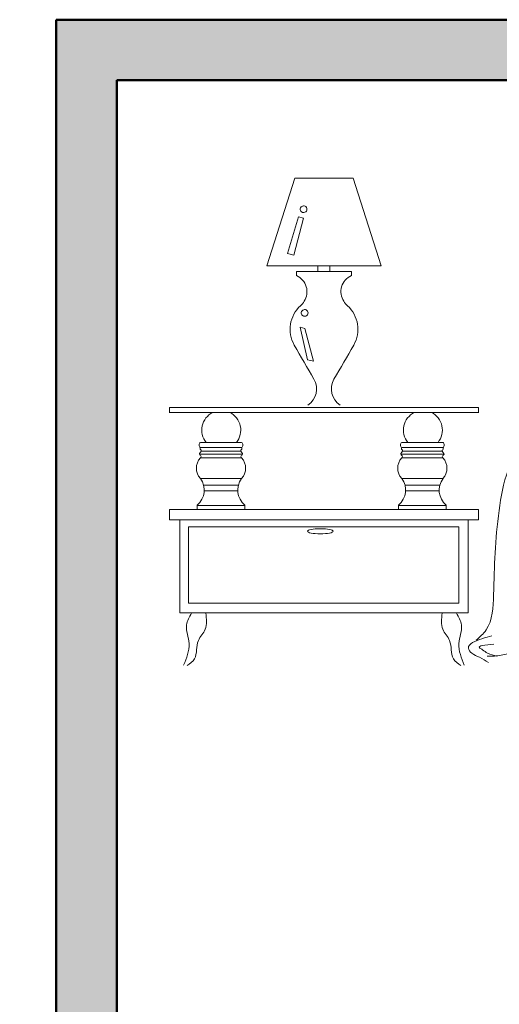
# Model space of a CAD drawing. Units: inches. Extents: x 1771 to 3025, y 319 to 889.
# Tile 9 of 35: x 1939 to 1978, y 713 to 795. Entities that reach past the tile are written whole.
import ezdxf

# ---------------------------------------------------------------- set-up
doc = ezdxf.new("R2010")
doc.units = ezdxf.units.IN
doc.header["$MEASUREMENT"] = 0
for name, color, linetype, lineweight in [('A-FURN', 8, 'Continuous', 18), ('A-WALL', 7, 'Continuous', 50), ('A-WALL-PATT', 254, 'Continuous', 13)]:
    doc.layers.add(name, color=color, linetype=linetype, lineweight=lineweight)

# ---------------------------------------------------------------- blocks, each defined once
blk = doc.blocks.new('A$C3F6F0378')
for p, q in [((188.6, 774.2), (242.7, 943.6)), ((356.2, 943.6), (242.7, 943.6)), ((410.4, 774.2), (356.2, 943.6)), ((229, 797.8), (250.3, 869.3)), ((259.4, 866.2), (241.2, 794.8)), ((250.3, 869.3), (259.4, 866.2)), ((241.2, 794.8), (229, 797.8)), ((410.4, 774.2), (188.6, 774.2)), ((246.2, 763), (246.2, 755.2)), ((246.2, 763), (246.2, 755.2)), ((352.5, 763), (246.2, 763)), ((287.7, 774.2), (287.7, 763)), ((311, 763), (287.7, 763)), ((311, 774.2), (311, 763)), ((352.5, 763), (352.5, 755.2)), ((352.5, 763), (352.5, 755.2)), ((253.5, 655.6), (262.6, 652.5)), ((267.2, 592.3), (253.5, 655.6)), ((262.6, 652.5), (279.4, 589.2)), ((279.4, 589.2), (267.2, 592.3)), ((598.4, 500), (0, 500)), ((0, 499.7), (0, 489.7)), ((598.4, 499.7), (598.4, 489.7)), ((598.4, 490), (0, 490)), ((140, 432.2), (60, 432.2)), ((140, 432.2), (60, 432.2)), ((140, 422.2), (60, 422.2)), ((529.9, 432.2), (449.9, 432.2)), ((529.9, 432.2), (449.9, 432.2)), ((529.9, 422.2), (449.9, 422.2)), ((141.9, 409.3), (58.1, 409.3)), ((140, 402.2), (60, 402.2)), ((138.2, 415.4), (61.8, 415.4)), ((531.8, 409.3), (447.9, 409.3)), ((529.9, 402.2), (449.9, 402.2)), ((528.1, 415.4), (451.7, 415.4)), ((140, 362.2), (60, 362.2)), ((133.7, 349.2), (66.3, 349.2)), ((529.9, 362.2), (449.9, 362.2)), ((523.5, 349.2), (456.2, 349.2)), ((132.4, 338.7), (67.5, 338.7)), ((522.3, 338.7), (457.4, 338.7)), ((53.7, 311), (53.7, 302.2)), ((146.3, 310.3), (53.7, 310.3)), ((146.3, 311), (146.3, 302.2)), ((443.6, 311), (443.6, 302.2)), ((536.1, 310.3), (443.6, 310.3)), ((536.1, 311), (536.1, 302.2)), ((0, 302.2), (0, 282.2)), ((598.4, 302.2), (0, 302.2)), ((80, 302.2), (120, 302.2)), ((80, 302.2), (130, 302.2)), ((469.9, 302.2), (509.9, 302.2)), ((469.9, 302.2), (519.9, 302.2)), ((598.4, 282.2), (598.4, 302.2)), ((598.4, 282.2), (0, 282.2)), ((20, 282.2), (20, 102.2)), ((37.2, 268.9), (560.2, 268.9)), ((37.2, 120.8), (37.2, 268.9)), ((560.2, 268.9), (560.2, 120.8)), ((578.4, 102.2), (578.4, 282.2)), ((560.2, 120.8), (37.2, 120.8)), ((20, 102.2), (578.4, 102.2))]:
    blk.add_line(p, q)
for centre, radius, start, end in [((259.7, 883.6), 6.48, 168.6084, 233.2112), ((259.7, 883.6), 6.49, 104.0344, 168.6084), ((259.6, 883.5), 6.42, 233.2112, 255.9722), ((260, 883.6), 6.51, 78.6968, 107.1924), ((259.7, 883.8), 6.69, 255.9722, 278.2688), ((259.7, 883.9), 6.81, 278.2688, 342.9026), ((260, 883.7), 6.5, 50.1648, 78.6968), ((260.1, 883.8), 6.35, 342.9026, 50.1648), ((232.6, 724.1), 33.9, 326.6744, 66.3416), ((366.1, 724.1), 33.9, 113.6584, 213.3256), ((231, 722.3), 34.4, 312.0366, 330.6067), ((367.7, 722.3), 34.4, 209.3933, 227.9634), ((295.2, 651.2), 61.5, 132.0366, 209.8723), ((261.7, 682.8), 6.49, 104.0344, 168.6084), ((262, 682.9), 6.51, 78.6968, 107.1924), ((262, 682.9), 6.5, 50.1648, 78.6968), ((262.1, 683), 6.35, 342.9026, 50.1648), ((303.6, 651.2), 61.5, 330.1277, 47.9634), ((261.7, 682.8), 6.48, 168.6084, 233.2112), ((261.6, 682.8), 6.42, 233.2112, 255.9722), ((261.7, 683), 6.69, 255.9722, 278.2688), ((261.7, 683.1), 6.81, 278.2688, 342.9026), ((9112.8, 5715.8), 10230.1, 209.87228, 210.29853), ((-8514, 5715.8), 10230.1, 329.70147, 330.12772), ((247.8, 535.9), 37.3, 302.5427, 30.2985), ((350.9, 535.9), 37.3, 149.7015, 237.4573), ((100.5, 456.1), 37.8, 115.9414, 219.2084), ((100.5, 456.1), 37.8, 320.7916, 64.0586), ((490.9, 456.1), 37.8, 115.9414, 219.2084), ((490.9, 456.1), 37.8, 320.7916, 64.0586), ((63.7, 427.2), 6.24, 126.78, 233.22), ((136.2, 427.2), 6.24, 306.78, 53.22), ((453.6, 427.2), 6.24, 126.78, 233.22), ((526.1, 427.2), 6.24, 306.78, 53.22), ((82, 382.2), 29.7, 137.7452, 222.2548), ((118, 382.2), 29.7, 317.7452, 42.2548), ((471.9, 382.2), 29.7, 137.7452, 222.2548), ((507.8, 382.2), 29.7, 317.7452, 42.2548), ((30.6, 339.8), 37, 308.7547, 37.2668), ((169.4, 339.8), 37, 142.7332, 231.2453), ((420.5, 339.8), 37, 308.7547, 37.2668), ((559.3, 339.8), 37, 142.7332, 231.2453)]:
    blk.add_arc(centre, radius, start, end)
blk.add_ellipse((292.3, 260.1), major_axis=(25, 0), ratio=0.2)
at = {"ltscale": 5}
for points, knots in [([(594.1, 49), (601.1, 55.3), (626, 78.1), (628.7, 172), (631.8, 287.1), (663.1, 436.6), (808.3, 475), (1037.5, 455.3), (1227.9, 458.5), (1322.1, 461.7)], [0, 0, 0, 0, 28.320233, 100.953775, 269.820348, 420.691469, 489.161544, 656.134073, 940.569207, 940.569207, 940.569207, 940.569207]), ([(624.2, 57.4), (618.3, 55.8), (603.1, 51.8), (572.2, 40.6), (586.5, 21.1), (602, 16.6), (612.3, 9.7), (617.8, 5.9)], [0, 0, 0, 0, 19.937155, 51.57724, 63.193909, 80.21631, 100.09061, 100.09061, 100.09061, 100.09061]), ([(628, 41.8), (612, 40.1), (592.4, 38.1), (608.5, 29.7), (617.4, 21.9), (627.8, 19.8), (634.3, 18.4)], [0, 0, 0, 0, 28.05485, 34.289435, 45.980108, 65.027556, 65.027556, 65.027556, 65.027556]), ([(615.5, 18.4), (620.3, 18.3), (633.7, 17.9), (664.9, 24.9), (717, 41.9), (776.4, 46.5), (816.6, 50.9), (832.8, 53.1), (835.5, 51), (835.9, 50.7)], [0, 0, 0, 0, 14.447875, 40.468341, 96.220884, 181.018327, 216.046098, 224.609189, 226.185962, 226.185962, 226.185962, 226.185962])]:
    blk.add_open_spline(points, degree=3, knots=knots, dxfattribs=at)
for points, knots in [([(60, 422.2), (59.5, 421), (58.6, 418.8), (63.4, 417.1), (60.1, 412.9), (56.2, 408.7), (63.1, 405.7), (60.8, 403.1), (60, 402.2)], [0, 0, 0, 0, 3.125, 6.207289, 10.622222, 14.901958, 20.470919, 23.596268, 23.596268, 23.596268, 23.596268]), ([(140, 422.2), (140.5, 421), (141.4, 418.8), (136.6, 417.1), (139.8, 412.9), (143.7, 408.7), (136.9, 405.7), (139.2, 403.1), (140, 402.2)], [0, 0, 0, 0, 3.125, 6.207289, 10.622222, 14.901958, 20.470919, 23.596268, 23.596268, 23.596268, 23.596268]), ([(449.9, 422.2), (449.4, 421), (448.5, 418.8), (453.2, 417.1), (450, 412.9), (446.1, 408.7), (453, 405.7), (450.7, 403.1), (449.9, 402.2)], [0, 0, 0, 0, 3.125, 6.207289, 10.622222, 14.901958, 20.470919, 23.596268, 23.596268, 23.596268, 23.596268]), ([(529.8, 422.2), (530.3, 421), (531.3, 418.8), (526.5, 417.1), (529.7, 412.9), (533.6, 408.7), (526.8, 405.7), (529, 403.1), (529.8, 402.2)], [0, 0, 0, 0, 3.125, 6.207289, 10.622222, 14.901958, 20.470919, 23.596268, 23.596268, 23.596268, 23.596268]), ([(42.9, 101.6), (38.6, 94.2), (28.1, 75.7), (43.8, 40.1), (33.3, 14.7), (27.7, 0.9)], [0, 0, 0, 0, 24.696996, 61.099524, 104.177437, 104.177437, 104.177437, 104.177437]), ([(70.4, 101.6), (71.9, 90.6), (74.7, 70.5), (49.8, 47.4), (55.7, 15.4), (39.9, 4), (34.3, 0)], [0, 0, 0, 0, 31.35672, 56.935761, 92.890491, 112.386558, 112.386558, 112.386558, 112.386558]), ([(528.3, 101.6), (526.8, 90.6), (524.1, 70.5), (549, 47.4), (543, 15.4), (558.9, 4), (564.5, 0)], [0, 0, 0, 0, 31.35672, 56.935761, 92.890491, 112.386558, 112.386558, 112.386558, 112.386558]), ([(555.9, 101.6), (560.2, 94.2), (570.6, 75.7), (554.9, 40.1), (565.4, 14.7), (571.1, 0.9)], [0, 0, 0, 0, 24.696996, 61.099524, 104.177437, 104.177437, 104.177437, 104.177437])]:
    blk.add_open_spline(points, degree=3, knots=knots)

msp = doc.modelspace()

# ---------------------------------------------------------------- hatches: boundary and pattern name
at = {"layer": 'A-WALL-PATT'}
h = msp.add_hatch(color=256, dxfattribs=at)
h.dxf.hatch_style = 1
h.paths.add_polyline_path([(1870.724, 888.634), (1799.724, 888.634), (1799.724, 878.634), (1870.724, 878.634)])
h.paths.add_polyline_path([(1968.767, 888.634), (1918.724, 888.634), (1918.724, 878.634), (1941.724, 878.634), (1941.724, 830.634), (1946.724, 830.634), (1946.724, 878.634), (1968.767, 878.634)])
h.paths.add_polyline_path([(2059.676, 888.634), (2016.767, 888.634), (2016.767, 878.634), (2037.724, 878.634), (2037.724, 794.634), (1941.724, 794.634), (1941.724, 758.634), (1941.724, 664.634), (1946.724, 664.634), (1946.724, 712), (1946.724, 789.634), (2054.724, 789.634), (2054.724, 794.634), (2042.325, 794.634), (2042.325, 798.62), (2042.325, 835.497), (2042.724, 878.634), (2059.676, 878.634)])
h.paths.add_polyline_path([(2100.724, 888.634), (2077.676, 888.634), (2077.676, 878.634), (2090.724, 878.634), (2090.724, 789.634), (2090.724, 768.608), (2100.724, 768.608)])
h.paths.add_polyline_path([(2100.724, 720.608), (2090.724, 720.608), (2090.724, 669.634), (1982.724, 669.634), (1982.724, 664.634), (2001.724, 664.634), (2001.724, 652.634), (2006.724, 652.634), (2006.724, 664.634), (2049.518, 664.634, -0.385549), (2050.522, 664.634), (2090.724, 664.634), (2090.724, 649.173), (2100.724, 649.173)])
edge = h.paths.add_edge_path()
edge.add_line((2100.724, 631.173), (2090.724, 631.173))
edge.add_line((2090.724, 631.173), (2090.724, 616.634))
edge.add_line((2090.724, 616.634), (2001.724, 616.634))
edge.add_line((2001.724, 616.634), (1982.724, 616.634))
edge.add_line((1982.724, 616.634), (1982.724, 611.634))
edge.add_line((1982.724, 611.634), (2024.672, 611.634))
edge.add_spline(control_points=[(2024.672, 611.634), (2027.581, 612.871), (2030.014, 613.313), (2032.469, 613.716)], knot_values=[484.321569, 484.321569, 484.321569, 484.321569, 625.498764, 625.498764, 625.498764, 625.498764], degree=3, periodic=0)
edge.add_line((2032.469, 613.716), (2033.205, 613.716))
edge.add_spline(control_points=[(2033.205, 613.716), (2035.66, 613.313), (2039.461, 612.871), (2042.204, 611.634)], knot_values=[484.321569, 484.321569, 484.321569, 484.321569, 625.498764, 625.498764, 625.498764, 625.498764], degree=3, periodic=0)
edge.add_line((2042.204, 611.634), (2090.724, 611.634))
edge.add_line((2090.724, 611.634), (2090.724, 581.106))
edge.add_line((2090.724, 581.106), (2100.724, 581.106))
edge.add_line((2100.724, 581.106), (2100.724, 631.173))
h.paths.add_polyline_path([(2100.724, 533.106), (2090.724, 533.106), (2090.724, 479.634), (1946.724, 479.634), (1946.724, 616.634), (1936.724, 616.634), (1936.724, 543.634), (1845.724, 543.634), (1845.724, 533.634), (1936.724, 533.634), (1936.724, 469.634), (2090.724, 469.634), (2090.724, 452.762), (2100.724, 452.762)])
h.paths.add_polyline_path([(2100.724, 404.762), (2090.724, 404.762), (2090.724, 393.634), (1936.724, 393.634), (1936.724, 383.634), (2100.724, 383.634)])
h.paths.add_polyline_path([(1905.724, 758.634), (1835.47, 758.634), (1835.47, 758.634), (1813.444, 758.634), (1809.724, 758.634), (1809.724, 842.589, -0.008336), (1808.421, 842.634), (1799.724, 842.634), (1799.724, 690.584), (1809.724, 690.584), (1809.724, 753.634), (1905.724, 753.634)])
h.paths.add_polyline_path([(1809.724, 642.584), (1799.724, 642.584), (1799.724, 533.634), (1809.724, 533.634), (1809.724, 581)])

# ---------------------------------------------------------------- linework, layer by layer
at = {"layer": 'A-WALL'}
for p, q in [((2037.724, 794.634), (1941.724, 794.634)), ((1941.724, 794.634), (1941.724, 758.634)), ((2054.724, 789.634), (1946.724, 789.634)), ((1946.724, 789.634), (1946.724, 669.634)), ((1941.724, 758.634), (1941.724, 664.634))]:
    msp.add_line(p, q, dxfattribs=at)

# ---------------------------------------------------------------- block references
at = {"layer": 'A-FURN', "xscale": 0.0427162254345911, "yscale": 0.0427162254345911, "zscale": 0.0427162254345911}
msp.add_blockref('A$C3F6F0378', (1951.078, 741.208), dxfattribs=at)

doc.saveas('drawing.dxf')
